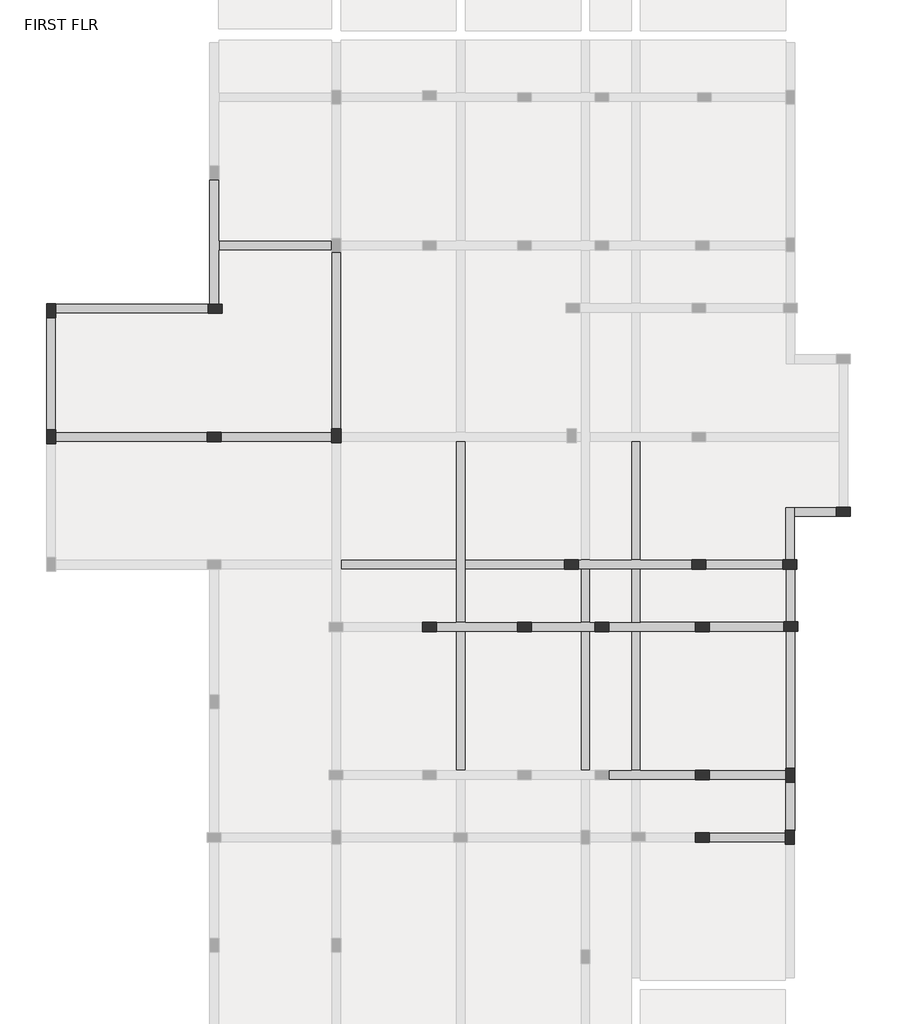
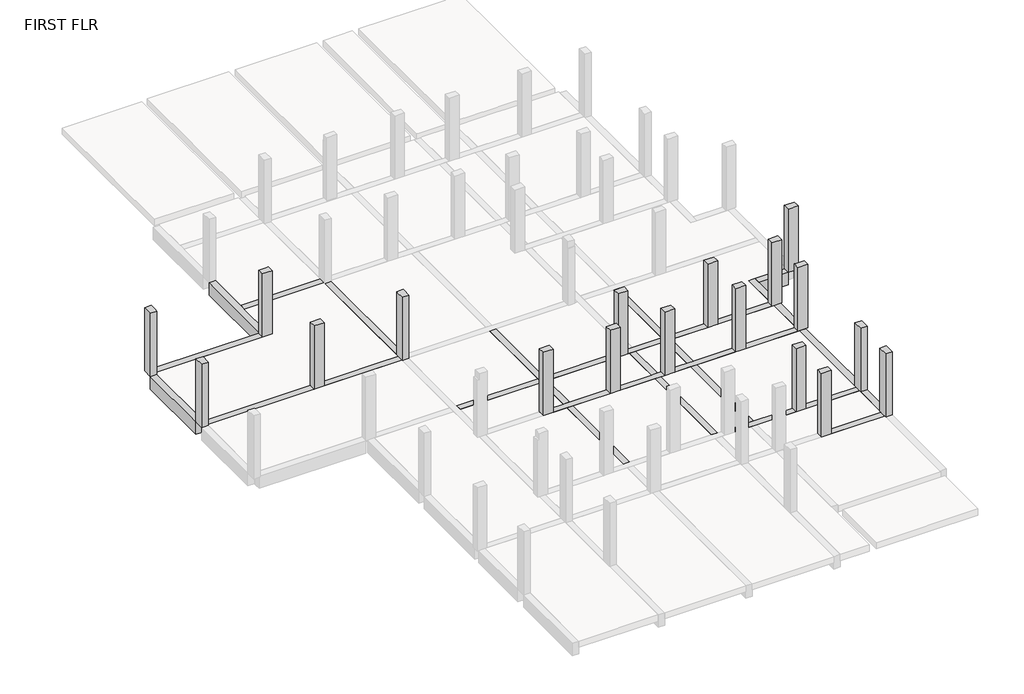
# One storey, part 3 of 5: 30 beams, 18 columns.
"""IFC4 building model written with IfcOpenShell, lengths in millimetres."""

from ifc_helpers import new_model, si_unit, frame, origin, place, context, project, spatial, polyline, outline, extrude, faceted_brep, element, save

model = new_model("IFC4")

# Units and contexts
model_context = context("Model", 3, world=origin())
ifc_project = project(units=[si_unit("LENGTHUNIT", "METRE", prefix="MILLI")], contexts=[model_context])

# Site, building, storey
site = spatial("IfcSite", under=ifc_project)
building = spatial("IfcBuilding", under=site)
storey = spatial("IfcBuildingStorey", under=building, Name="FIRST FLR", Elevation=3000.0)

# Beams
placement = place(None, origin())
element("IfcBeam", 1, ObjectType="M_Concrete-Rectangular Beam : 300 x 600mm", at=placement, inside=storey, context=model_context, shape_type="Brep", body=[
    faceted_brep([(-5888.8105653, 9367.5252033, 3000.0), (-5888.8105653, 5367.5252033, 3000.0), (-5588.8105653, 5367.5252033, 3000.0), (-5588.8105653, 7099.7076276, 3000.0), (-5588.8105653, 7399.7076276, 3000.0), (-5588.8105653, 9367.5252033, 3000.0), (-5888.8105653, 9367.5252033, 2400.0), (-5888.8105653, 5367.5252033, 2400.0), (-5588.8105653, 9367.5252033, 2400.0), (-5588.8105653, 7399.7076276, 2400.0), (-5588.8105653, 7099.7076276, 2400.0), (-5588.8105653, 5367.5252033, 2400.0), (-5588.8105653, 9367.5252033, 2700.0), (-5588.8105653, 5367.5252033, 2700.0)], [[[0, 1, 2, 3, 4, 5]], [[1, 0, 6, 7]], [[7, 6, 8, 9, 10, 11]], [[11, 10, 9, 8, 12, 5, 4, 3, 2, 13]], [[8, 6, 0, 5, 12]], [[2, 1, 7, 11, 13]]]),
])
element("IfcBeam", 2, ObjectType="M_Concrete-Rectangular Beam : 300 x 600mm", at=placement, inside=storey, context=model_context, shape_type="Brep", body=[
    faceted_brep([(-5943.8105653, 5067.6057249, 3000.0), (-5943.8105653, 5367.6057249, 3000.0), (-10828.8105653, 5367.6057249, 3000.0), (-10828.8105653, 5067.6057249, 3000.0), (-5943.8105653, 5367.6057249, 2400.0), (-10828.8105653, 5367.6057249, 2400.0), (-5943.8105653, 5067.6057249, 2400.0), (-10828.8105653, 5067.6057249, 2400.0), (-10828.8105653, 5067.6057249, 2700.0), (-5943.8105653, 5067.6057249, 2700.0)], [[[0, 1, 2, 3]], [[1, 4, 5, 2]], [[4, 6, 7, 5]], [[0, 3, 8, 7, 6, 9]], [[6, 4, 1, 0, 9]], [[3, 2, 5, 7, 8]]]),
])
element("IfcBeam", 3, ObjectType="M_Concrete-Rectangular Beam : 300 x 600mm", at=placement, inside=storey, context=model_context, shape_type="SweptSolid", body=[
    extrude(outline(polyline([(-10828.8105653, 1326.1713929), (-11128.8105653, 1326.1713929), (-11128.8105653, 4932.6057249), (-10828.8105653, 4932.6057249), (-10828.8105653, 1326.1713929)])), frame((0.0, 0.0, 2400.0), z_axis=(0.0, 0.0, 1.0), x_axis=(1.0, 0.0, 0.0)), (0.0, 0.0, 1.0), 600.0),
])
element("IfcBeam", 4, ObjectType="M_Concrete-Rectangular Beam : 300 x 600mm", at=placement, inside=storey, context=model_context, shape_type="SweptSolid", body=[
    extrude(outline(polyline([(12619.1163908, -9982.1078267), (12919.1163908, -9982.1078267), (12919.1163908, -11537.8970059), (12899.1163908, -11537.8970059), (12899.1163908, -11532.8970059), (12619.1163908, -11532.8970059), (12619.1163908, -9982.1078267)])), frame((0.0, 0.0, 2400.0), z_axis=(0.0, 0.0, 1.0), x_axis=(1.0, 0.0, 0.0)), (0.0, 0.0, 1.0), 600.0),
])
element("IfcBeam", 5, ObjectType="M_Concrete-Rectangular Beam : 300 x 600mm", at=placement, inside=storey, context=model_context, shape_type="Brep", body=[
    faceted_brep([(12619.1163908, -5144.3229916, 3000.0), (12919.1163908, -5144.3229916, 3000.0), (12919.1163908, -5144.3229916, 2400.0), (12619.1163908, -5144.3229916, 2400.0), (12619.1163908, -5151.6229916, 3000.0), (12619.1163908, -9532.1078267, 3000.0), (12919.1163908, -9532.1078267, 3000.0), (12919.1163908, -9532.1078267, 2400.0), (12619.1163908, -9532.1078267, 2400.0), (12619.1163908, -5151.6229916, 2400.0), (12619.1163908, -9532.1078267, 2700.0)], [[[0, 1, 2, 3]], [[1, 0, 4, 5, 6]], [[2, 1, 6, 7]], [[3, 2, 7, 8, 9]], [[0, 3, 9, 8, 10, 5, 4]], [[8, 7, 6, 5, 10]]]),
])
element("IfcBeam", 6, ObjectType="M_Concrete-Rectangular Beam : 300 x 600mm", at=placement, inside=storey, context=model_context, shape_type="Brep", body=[
    faceted_brep([(12619.1163908, -4818.9229916, 2400.0), (12919.1163908, -4818.9229916, 2400.0), (12919.1163908, -4818.9229916, 3000.0), (12619.1163908, -4818.9229916, 3000.0), (12619.1163908, -4818.9229916, 2700.0), (12919.1163908, -3139.4535766, 3000.0), (12619.1163908, -3139.4535766, 3000.0), (12919.1163908, -3139.4535766, 2400.0), (12619.1163908, -3139.4535766, 2400.0), (12619.1163908, -3139.4535766, 2700.0)], [[[0, 1, 2, 3, 4]], [[3, 2, 5, 6]], [[2, 1, 7, 5]], [[1, 0, 8, 7]], [[3, 6, 9, 8, 0, 4]], [[6, 5, 7, 8, 9]]]),
])
element("IfcBeam", 7, ObjectType="M_Concrete-Rectangular Beam : 300 x 600mm", at=placement, inside=storey, context=model_context, shape_type="Brep", body=[
    faceted_brep([(12599.1163908, -2839.4535766, 3000.0), (12899.1163908, -2839.4535766, 3000.0), (12899.1163908, -1448.8286071, 3000.0), (12899.1163908, -1148.8286071, 3000.0), (12599.1163908, -1148.8286071, 3000.0), (12899.1163908, -2839.4535766, 2400.0), (12899.1163908, -1448.8286071, 2400.0), (12899.1163908, -1148.8286071, 2400.0), (12899.1163908, -1148.8286071, 2700.0), (12599.1163908, -2839.4535766, 2400.0), (12599.1163908, -1148.8286071, 2400.0), (12599.1163908, -1148.8286071, 2700.0), (12599.1163908, -2839.4535766, 2700.0)], [[[0, 1, 2, 3, 4]], [[1, 5, 6, 7, 8, 3, 2]], [[5, 9, 10, 7, 6]], [[0, 4, 11, 10, 9, 12]], [[9, 5, 1, 0, 12]], [[4, 3, 8, 7, 10, 11]]]),
])
element("IfcBeam", 8, ObjectType="M_Concrete-Rectangular Beam : 300 x 600mm", at=placement, inside=storey, context=model_context, shape_type="Brep", body=[
    faceted_brep([(14244.1163908, -1448.8286071, 3000.0), (14244.1163908, -1148.8286071, 3000.0), (12899.1163908, -1148.8286071, 3000.0), (12899.1163908, -1448.8286071, 3000.0), (14244.1163908, -1148.8286071, 2700.0), (14244.1163908, -1148.8286071, 2400.0), (12899.1163908, -1148.8286071, 2400.0), (12899.1163908, -1148.8286071, 2700.0), (14244.1163908, -1448.8286071, 2400.0), (12899.1163908, -1448.8286071, 2400.0)], [[[0, 1, 2, 3]], [[2, 1, 4, 5, 6, 7]], [[5, 8, 9, 6]], [[8, 0, 3, 9]], [[0, 8, 5, 4, 1]], [[3, 2, 7, 6, 9]]]),
])
element("IfcBeam", 9, ObjectType="M_Concrete-Rectangular Beam : 300 x 600mm", at=placement, inside=storey, context=model_context, shape_type="Brep", body=[
    faceted_brep([(-1671.7865686, 7024.7076276, 3000.0), (-1971.7865686, 7024.7076276, 3000.0), (-1971.7865686, 1366.1713929, 3000.0), (-1671.7865686, 1366.1713929, 3000.0), (-1971.7865686, 7024.7076276, 2700.0), (-1971.7865686, 7024.7076276, 2400.0), (-1971.7865686, 1366.1713929, 2400.0), (-1971.7865686, 1366.1713929, 2700.0), (-1671.7865686, 7024.7076276, 2400.0), (-1671.7865686, 1366.1713929, 2400.0), (-1671.7865686, 1366.1713929, 2700.0), (-1671.7865686, 7024.7076276, 2700.0)], [[[0, 1, 2, 3]], [[2, 1, 4, 5, 6, 7]], [[5, 8, 9, 6]], [[0, 3, 10, 9, 8, 11]], [[1, 0, 11, 8, 5, 4]], [[3, 2, 7, 6, 9, 10]]]),
])
element("IfcBeam", 10, ObjectType="M_Concrete-Rectangular Beam : 300 x 600mm", at=placement, inside=storey, context=model_context, shape_type="Brep", body=[
    faceted_brep([(-1971.7865686, 7099.7076276, 3000.0), (-1971.7865686, 7399.7076276, 3000.0), (-5588.8105653, 7399.7076276, 3000.0), (-5588.8105653, 7099.7076276, 3000.0), (-5588.8105653, 7099.7076276, 2700.0), (-5588.8105653, 7099.7076276, 2400.0), (-1971.7865686, 7099.7076276, 2400.0), (-1971.7865686, 7099.7076276, 2700.0), (-1971.7865686, 7399.7076276, 2400.0), (-5588.8105653, 7399.7076276, 2400.0), (-1971.7865686, 7399.7076276, 2700.0), (-5588.8105653, 7399.7076276, 2700.0)], [[[0, 1, 2, 3]], [[0, 3, 4, 5, 6, 7]], [[8, 6, 5, 9]], [[2, 1, 10, 8, 9, 11]], [[1, 0, 7, 6, 8, 10]], [[3, 2, 11, 9, 5, 4]]]),
])
element("IfcBeam", 11, ObjectType="M_Concrete-Rectangular Beam : 300 x 600mm", at=placement, inside=storey, context=model_context, shape_type="Brep", body=[
    faceted_brep([(-10828.8105653, 1251.1713929, 3000.0), (-10828.8105653, 951.1713929, 3000.0), (-5963.8105653, 951.1713929, 3000.0), (-5963.8105653, 1251.1713929, 3000.0), (-10828.8105653, 951.1713929, 2700.0), (-10828.8105653, 951.1713929, 2400.0), (-5963.8105653, 951.1713929, 2400.0), (-5963.8105653, 951.1713929, 2700.0), (-10828.8105653, 1251.1713929, 2400.0), (-5963.8105653, 1251.1713929, 2400.0), (-5963.8105653, 1251.1713929, 2700.0), (-10828.8105653, 1251.1713929, 2700.0)], [[[0, 1, 2, 3]], [[2, 1, 4, 5, 6, 7]], [[5, 8, 9, 6]], [[0, 3, 10, 9, 8, 11]], [[1, 0, 11, 8, 5, 4]], [[3, 2, 7, 6, 9, 10]]]),
])
element("IfcBeam", 12, ObjectType="M_Concrete-Rectangular Beam : 300 x 600mm", at=placement, inside=storey, context=model_context, shape_type="Brep", body=[
    faceted_brep([(-5513.8105653, 1251.1713929, 3000.0), (-5513.8105653, 951.1713929, 3000.0), (-1971.7865686, 951.1713929, 3000.0), (-1971.7865686, 1251.1713929, 3000.0), (-5513.8105653, 951.1713929, 2700.0), (-5513.8105653, 951.1713929, 2400.0), (-1971.7865686, 951.1713929, 2400.0), (-1971.7865686, 951.1713929, 2700.0), (-5513.8105653, 1251.1713929, 2400.0), (-1971.7865686, 1251.1713929, 2400.0), (-1971.7865686, 1251.1713929, 2700.0), (-5513.8105653, 1251.1713929, 2700.0)], [[[0, 1, 2, 3]], [[2, 1, 4, 5, 6, 7]], [[5, 8, 9, 6]], [[0, 3, 10, 9, 8, 11]], [[1, 0, 11, 8, 5, 4]], [[3, 2, 7, 6, 9, 10]]]),
])
element("IfcBeam", 13, ObjectType="M_Concrete-Rectangular Beam : 300 x 600mm", at=placement, inside=storey, context=model_context, shape_type="Brep", body=[
    faceted_brep([(9601.8679014, -3139.4535766, 3000.0), (9601.8679014, -2839.4535766, 3000.0), (7956.8679014, -2839.4535766, 3000.0), (7656.8679014, -2839.4535766, 3000.0), (6332.5248054, -2839.4535766, 3000.0), (6032.5248054, -2839.4535766, 3000.0), (5967.5248054, -2839.4535766, 3000.0), (5967.5248054, -3139.4535766, 3000.0), (6032.5248054, -3139.4535766, 3000.0), (6332.5248054, -3139.4535766, 3000.0), (7656.8679014, -3139.4535766, 3000.0), (7956.8679014, -3139.4535766, 3000.0), (5967.5248054, -3139.4535766, 2400.0), (6032.5248054, -3139.4535766, 2400.0), (6332.5248054, -3139.4535766, 2400.0), (7656.8679014, -3139.4535766, 2400.0), (7956.8679014, -3139.4535766, 2400.0), (9601.8679014, -3139.4535766, 2400.0), (9601.8679014, -3139.4535766, 2700.0), (5967.5248054, -3139.4535766, 2700.0), (9601.8679014, -2839.4535766, 2400.0), (5967.5248054, -2839.4535766, 2400.0), (6032.5248054, -2839.4535766, 2400.0), (6332.5248054, -2839.4535766, 2400.0), (7656.8679014, -2839.4535766, 2400.0), (7956.8679014, -2839.4535766, 2400.0), (5967.5248054, -2839.4535766, 2700.0), (9601.8679014, -2839.4535766, 2700.0)], [[[0, 1, 2, 3, 4, 5, 6, 7, 8, 9, 10, 11]], [[12, 13, 14, 15, 16, 17, 18, 0, 11, 10, 9, 8, 7, 19]], [[20, 17, 16, 15, 14, 13, 12, 21, 22, 23, 24, 25]], [[20, 25, 24, 23, 22, 21, 26, 6, 5, 4, 3, 2, 1, 27]], [[1, 0, 18, 17, 20, 27]], [[7, 6, 26, 21, 12, 19]]]),
])
element("IfcBeam", 14, ObjectType="M_Concrete-Rectangular Beam : 300 x 600mm", at=placement, inside=storey, context=model_context, shape_type="Brep", body=[
    faceted_brep([(12524.1163908, -3139.4535766, 3000.0), (12524.1163908, -2839.4535766, 3000.0), (10051.8679014, -2839.4535766, 3000.0), (10051.8679014, -3139.4535766, 3000.0), (10051.8679014, -3139.4535766, 2700.0), (10051.8679014, -3139.4535766, 2400.0), (12524.1163908, -3139.4535766, 2400.0), (12524.1163908, -3139.4535766, 2700.0), (12524.1163908, -2839.4535766, 2400.0), (10051.8679014, -2839.4535766, 2400.0), (12524.1163908, -2839.4535766, 2700.0), (10051.8679014, -2839.4535766, 2700.0)], [[[0, 1, 2, 3]], [[0, 3, 4, 5, 6, 7]], [[8, 6, 5, 9]], [[2, 1, 10, 8, 9, 11]], [[1, 0, 7, 6, 8, 10]], [[3, 2, 11, 9, 5, 4]]]),
])
element("IfcBeam", 15, ObjectType="M_Concrete-Rectangular Beam : 300 x 600mm", at=placement, inside=storey, context=model_context, shape_type="Brep", body=[
    faceted_brep([(1399.7296816, -4851.6229916, 3000.0), (1399.7296816, -5151.6229916, 3000.0), (2024.7296816, -5151.6229916, 3000.0), (2324.7296816, -5151.6229916, 3000.0), (3997.5248054, -5151.6229916, 3000.0), (3997.5248054, -4851.6229916, 3000.0), (2324.7296816, -4851.6229916, 3000.0), (2024.7296816, -4851.6229916, 3000.0), (1399.7296816, -5151.6229916, 2400.0), (2024.7296816, -5151.6229916, 2400.0), (2324.7296816, -5151.6229916, 2400.0), (3997.5248054, -5151.6229916, 2400.0), (3997.5248054, -5151.6229916, 2700.0), (1399.7296816, -5151.6229916, 2700.0), (1399.7296816, -4851.6229916, 2400.0), (2024.7296816, -4851.6229916, 2400.0), (2324.7296816, -4851.6229916, 2400.0), (3997.5248054, -4851.6229916, 2400.0), (1399.7296816, -4851.6229916, 2700.0), (3997.5248054, -4851.6229916, 2700.0)], [[[0, 1, 2, 3, 4, 5, 6, 7]], [[8, 9, 10, 11, 12, 4, 3, 2, 1, 13]], [[8, 14, 15, 16, 17, 11, 10, 9]], [[17, 16, 15, 14, 18, 0, 7, 6, 5, 19]], [[1, 0, 18, 14, 8, 13]], [[5, 4, 12, 11, 17, 19]]]),
])
element("IfcBeam", 16, ObjectType="M_Concrete-Rectangular Beam : 300 x 600mm", at=placement, inside=storey, context=model_context, shape_type="Brep", body=[
    faceted_brep([(4447.5248054, -4851.6229916, 3000.0), (4447.5248054, -5151.6229916, 3000.0), (6032.5248054, -5151.6229916, 3000.0), (6332.5248054, -5151.6229916, 3000.0), (6481.8679014, -5151.6229916, 3000.0), (6481.8679014, -4851.6229916, 3000.0), (6332.5248054, -4851.6229916, 3000.0), (6032.5248054, -4851.6229916, 3000.0), (4447.5248054, -5151.6229916, 2400.0), (6032.5248054, -5151.6229916, 2400.0), (6332.5248054, -5151.6229916, 2400.0), (6481.8679014, -5151.6229916, 2400.0), (6481.8679014, -5151.6229916, 2700.0), (4447.5248054, -5151.6229916, 2700.0), (4447.5248054, -4851.6229916, 2400.0), (6032.5248054, -4851.6229916, 2400.0), (6332.5248054, -4851.6229916, 2400.0), (6481.8679014, -4851.6229916, 2400.0), (4447.5248054, -4851.6229916, 2700.0)], [[[0, 1, 2, 3, 4, 5, 6, 7]], [[8, 9, 10, 11, 12, 4, 3, 2, 1, 13]], [[8, 14, 15, 16, 17, 11, 10, 9]], [[17, 16, 15, 14, 18, 0, 7, 6, 5]], [[1, 0, 18, 14, 8, 13]], [[5, 4, 12, 11, 17]]]),
])
element("IfcBeam", 17, ObjectType="M_Concrete-Rectangular Beam : 300 x 600mm", at=placement, inside=storey, context=model_context, shape_type="Brep", body=[
    faceted_brep([(6931.8679014, -4851.6229916, 3000.0), (6931.8679014, -5151.6229916, 3000.0), (7656.8679014, -5151.6229916, 3000.0), (7956.8679014, -5151.6229916, 3000.0), (9721.8679014, -5151.6229916, 3000.0), (9721.8679014, -4851.6229916, 3000.0), (7956.8679014, -4851.6229916, 3000.0), (7656.8679014, -4851.6229916, 3000.0), (6931.8679014, -5151.6229916, 2400.0), (7656.8679014, -5151.6229916, 2400.0), (7956.8679014, -5151.6229916, 2400.0), (9721.8679014, -5151.6229916, 2400.0), (9721.8679014, -5151.6229916, 2700.0), (6931.8679014, -5151.6229916, 2700.0), (6931.8679014, -4851.6229916, 2400.0), (7656.8679014, -4851.6229916, 2400.0), (7956.8679014, -4851.6229916, 2400.0), (9721.8679014, -4851.6229916, 2400.0)], [[[0, 1, 2, 3, 4, 5, 6, 7]], [[8, 9, 10, 11, 12, 4, 3, 2, 1, 13]], [[8, 14, 15, 16, 17, 11, 10, 9]], [[14, 0, 7, 6, 5, 17, 16, 15]], [[1, 0, 14, 8, 13]], [[5, 4, 12, 11, 17]]]),
])
element("IfcBeam", 18, ObjectType="M_Concrete-Rectangular Beam : 300 x 600mm", at=placement, inside=storey, context=model_context, shape_type="Brep", body=[
    faceted_brep([(12599.1163908, -11907.8970059, 3000.0), (12599.1163908, -11607.8970059, 3000.0), (10171.8679014, -11607.8970059, 3000.0), (10171.8679014, -11907.8970059, 3000.0), (10171.8679014, -11907.8970059, 2700.0), (10171.8679014, -11907.8970059, 2400.0), (12599.1163908, -11907.8970059, 2400.0), (12599.1163908, -11907.8970059, 2700.0), (12599.1163908, -11607.8970059, 2400.0), (10171.8679014, -11607.8970059, 2400.0), (12599.1163908, -11607.8970059, 2700.0), (10171.8679014, -11607.8970059, 2700.0)], [[[0, 1, 2, 3]], [[0, 3, 4, 5, 6, 7]], [[8, 6, 5, 9]], [[2, 1, 10, 8, 9, 11]], [[1, 0, 7, 6, 8, 10]], [[3, 2, 11, 9, 5, 4]]]),
])
element("IfcBeam", 19, ObjectType="M_Concrete-Rectangular Beam : 300 x 600mm", at=placement, inside=storey, context=model_context, shape_type="Brep", body=[
    faceted_brep([(6931.8679014, -9607.1078267, 3000.0), (6931.8679014, -9907.1078267, 3000.0), (7656.8679014, -9907.1078267, 3000.0), (7956.8679014, -9907.1078267, 3000.0), (9721.8679014, -9907.1078267, 3000.0), (9721.8679014, -9607.1078267, 3000.0), (7956.8679014, -9607.1078267, 3000.0), (7656.8679014, -9607.1078267, 3000.0), (6931.8679014, -9907.1078267, 2400.0), (7656.8679014, -9907.1078267, 2400.0), (7956.8679014, -9907.1078267, 2400.0), (9721.8679014, -9907.1078267, 2400.0), (9721.8679014, -9907.1078267, 2700.0), (6931.8679014, -9907.1078267, 2700.0), (6931.8679014, -9607.1078267, 2400.0), (7656.8679014, -9607.1078267, 2400.0), (7956.8679014, -9607.1078267, 2400.0), (9721.8679014, -9607.1078267, 2400.0), (6931.8679014, -9607.1078267, 2700.0), (9721.8679014, -9607.1078267, 2700.0)], [[[0, 1, 2, 3, 4, 5, 6, 7]], [[8, 9, 10, 11, 12, 4, 3, 2, 1, 13]], [[8, 14, 15, 16, 17, 11, 10, 9]], [[17, 16, 15, 14, 18, 0, 7, 6, 5, 19]], [[1, 0, 18, 14, 8, 13]], [[5, 4, 12, 11, 17, 19]]]),
])
element("IfcBeam", 20, ObjectType="M_Concrete-Rectangular Beam : 300 x 600mm", at=placement, inside=storey, context=model_context, shape_type="Brep", body=[
    faceted_brep([(10171.8679014, -9607.1078267, 3000.0), (10171.8679014, -9907.1078267, 3000.0), (12599.1163908, -9907.1078267, 3000.0), (12619.1163908, -9907.1078267, 3000.0), (12619.1163908, -9607.1078267, 3000.0), (10171.8679014, -9907.1078267, 2400.0), (12619.1163908, -9907.1078267, 2400.0), (10171.8679014, -9907.1078267, 2700.0), (10171.8679014, -9607.1078267, 2400.0), (12619.1163908, -9607.1078267, 2400.0), (12619.1163908, -9607.1078267, 2700.0), (10171.8679014, -9607.1078267, 2700.0)], [[[0, 1, 2, 3, 4]], [[5, 6, 3, 2, 1, 7]], [[5, 8, 9, 6]], [[0, 4, 10, 9, 8, 11]], [[1, 0, 11, 8, 5, 7]], [[4, 3, 6, 9, 10]]]),
])
element("IfcBeam", 21, ObjectType="M_Concrete-Rectangular Beam : 300 x 600mm", at=placement, inside=storey, context=model_context, shape_type="Brep", body=[
    faceted_brep([(-1671.7865686, -2839.4535766, 3000.0), (-1671.7865686, -3139.4535766, 3000.0), (2024.7296816, -3139.4535766, 3000.0), (2024.7296816, -2839.4535766, 3000.0), (-1671.7865686, -3139.4535766, 2700.0), (-1671.7865686, -3139.4535766, 2400.0), (2024.7296816, -3139.4535766, 2400.0), (2024.7296816, -3139.4535766, 2700.0), (-1671.7865686, -2839.4535766, 2400.0), (2024.7296816, -2839.4535766, 2400.0), (2024.7296816, -2839.4535766, 2700.0), (-1671.7865686, -2839.4535766, 2700.0)], [[[0, 1, 2, 3]], [[2, 1, 4, 5, 6, 7]], [[5, 8, 9, 6]], [[0, 3, 10, 9, 8, 11]], [[1, 0, 11, 8, 5, 4]], [[3, 2, 7, 6, 9, 10]]]),
])
element("IfcBeam", 22, ObjectType="M_Concrete-Rectangular Beam : 300 x 600mm", at=placement, inside=storey, context=model_context, shape_type="Brep", body=[
    faceted_brep([(6332.5248054, -3139.4535766, 3000.0), (6032.5248054, -3139.4535766, 3000.0), (6032.5248054, -4851.6229916, 3000.0), (6332.5248054, -4851.6229916, 3000.0), (6032.5248054, -3139.4535766, 2700.0), (6032.5248054, -3139.4535766, 2400.0), (6032.5248054, -4851.6229916, 2400.0), (6032.5248054, -4851.6229916, 2700.0), (6332.5248054, -3139.4535766, 2400.0), (6332.5248054, -4851.6229916, 2400.0), (6332.5248054, -3139.4535766, 2700.0), (6332.5248054, -4851.6229916, 2700.0)], [[[0, 1, 2, 3]], [[2, 1, 4, 5, 6, 7]], [[5, 8, 9, 6]], [[8, 10, 0, 3, 11, 9]], [[1, 0, 10, 8, 5, 4]], [[3, 2, 7, 6, 9, 11]]]),
])
element("IfcBeam", 23, ObjectType="M_Concrete-Rectangular Beam : 300 x 600mm", at=placement, inside=storey, context=model_context, shape_type="Brep", body=[
    faceted_brep([(7956.8679014, -3139.4535766, 3000.0), (7656.8679014, -3139.4535766, 3000.0), (7656.8679014, -4851.6229916, 3000.0), (7956.8679014, -4851.6229916, 3000.0), (7956.8679014, -4831.6229916, 3000.0), (7656.8679014, -3139.4535766, 2700.0), (7656.8679014, -3139.4535766, 2400.0), (7656.8679014, -4851.6229916, 2400.0), (7656.8679014, -4851.6229916, 2700.0), (7956.8679014, -3139.4535766, 2400.0), (7956.8679014, -4851.6229916, 2400.0), (7956.8679014, -3139.4535766, 2700.0)], [[[0, 1, 2, 3, 4]], [[1, 5, 6, 7, 8, 2]], [[6, 9, 10, 7]], [[10, 9, 11, 0, 4, 3]], [[1, 0, 11, 9, 6, 5]], [[3, 2, 8, 7, 10]]]),
])
element("IfcBeam", 24, ObjectType="M_Concrete-Rectangular Beam : 300 x 600mm", at=placement, inside=storey, context=model_context, shape_type="Brep", body=[
    faceted_brep([(2324.7296816, -5151.6229916, 3000.0), (2024.7296816, -5151.6229916, 3000.0), (2024.7296816, -9607.1078267, 3000.0), (2324.7296816, -9607.1078267, 3000.0), (2024.7296816, -5151.6229916, 2700.0), (2024.7296816, -5151.6229916, 2400.0), (2024.7296816, -9607.1078267, 2400.0), (2024.7296816, -9607.1078267, 2700.0), (2324.7296816, -5151.6229916, 2400.0), (2324.7296816, -9607.1078267, 2400.0), (2324.7296816, -9607.1078267, 2700.0), (2324.7296816, -5151.6229916, 2700.0)], [[[0, 1, 2, 3]], [[2, 1, 4, 5, 6, 7]], [[5, 8, 9, 6]], [[0, 3, 10, 9, 8, 11]], [[1, 0, 11, 8, 5, 4]], [[3, 2, 7, 6, 9, 10]]]),
])
element("IfcBeam", 25, ObjectType="M_Concrete-Rectangular Beam : 300 x 600mm", at=placement, inside=storey, context=model_context, shape_type="Brep", body=[
    faceted_brep([(6332.5248054, -5151.6229916, 3000.0), (6032.5248054, -5151.6229916, 3000.0), (6032.5248054, -9607.1078267, 3000.0), (6332.5248054, -9607.1078267, 3000.0), (6032.5248054, -5151.6229916, 2700.0), (6032.5248054, -5151.6229916, 2400.0), (6032.5248054, -9607.1078267, 2400.0), (6032.5248054, -9607.1078267, 2700.0), (6332.5248054, -5151.6229916, 2400.0), (6332.5248054, -9607.1078267, 2400.0), (6332.5248054, -9607.1078267, 2700.0), (6332.5248054, -5151.6229916, 2700.0)], [[[0, 1, 2, 3]], [[2, 1, 4, 5, 6, 7]], [[5, 8, 9, 6]], [[0, 3, 10, 9, 8, 11]], [[1, 0, 11, 8, 5, 4]], [[3, 2, 7, 6, 9, 10]]]),
])
element("IfcBeam", 26, ObjectType="M_Concrete-Rectangular Beam : 300 x 600mm", at=placement, inside=storey, context=model_context, shape_type="Brep", body=[
    faceted_brep([(7956.8679014, -5151.6229916, 3000.0), (7656.8679014, -5151.6229916, 3000.0), (7656.8679014, -9607.1078267, 3000.0), (7956.8679014, -9607.1078267, 3000.0), (7656.8679014, -5151.6229916, 2700.0), (7656.8679014, -5151.6229916, 2400.0), (7656.8679014, -9607.1078267, 2400.0), (7656.8679014, -9607.1078267, 2700.0), (7956.8679014, -5151.6229916, 2400.0), (7956.8679014, -9607.1078267, 2400.0), (7956.8679014, -9607.1078267, 2700.0), (7956.8679014, -5151.6229916, 2700.0)], [[[0, 1, 2, 3]], [[2, 1, 4, 5, 6, 7]], [[5, 8, 9, 6]], [[0, 3, 10, 9, 8, 11]], [[1, 0, 11, 8, 5, 4]], [[3, 2, 7, 6, 9, 10]]]),
])
element("IfcBeam", 27, ObjectType="M_Concrete-Rectangular Beam : 300 x 600mm", at=placement, inside=storey, context=model_context, shape_type="Brep", body=[
    faceted_brep([(2024.7296816, -4851.6229916, 3000.0), (2324.7296816, -4851.6229916, 3000.0), (2324.7296816, -3139.4535766, 3000.0), (2324.7296816, -2839.4535766, 3000.0), (2324.7296816, 951.1713929, 3000.0), (2024.7296816, 951.1713929, 3000.0), (2024.7296816, -2839.4535766, 3000.0), (2024.7296816, -3139.4535766, 3000.0), (2024.7296816, 951.1713929, 2400.0), (2024.7296816, -2839.4535766, 2400.0), (2024.7296816, -3139.4535766, 2400.0), (2024.7296816, -4851.6229916, 2400.0), (2024.7296816, -4851.6229916, 2700.0), (2024.7296816, 951.1713929, 2700.0), (2324.7296816, -4851.6229916, 2400.0), (2324.7296816, 951.1713929, 2400.0), (2324.7296816, -2839.4535766, 2400.0), (2324.7296816, -3139.4535766, 2400.0), (2324.7296816, 951.1713929, 2700.0), (2324.7296816, -4851.6229916, 2700.0)], [[[0, 1, 2, 3, 4, 5, 6, 7]], [[8, 9, 10, 11, 12, 0, 7, 6, 5, 13]], [[14, 11, 10, 9, 8, 15, 16, 17]], [[14, 17, 16, 15, 18, 4, 3, 2, 1, 19]], [[1, 0, 12, 11, 14, 19]], [[5, 4, 18, 15, 8, 13]]]),
])
element("IfcBeam", 28, ObjectType="M_Concrete-Rectangular Beam : 300 x 600mm", at=placement, inside=storey, context=model_context, shape_type="Brep", body=[
    faceted_brep([(5517.5248054, -3139.4535766, 3000.0), (5517.5248054, -2839.4535766, 3000.0), (2324.7296816, -2839.4535766, 3000.0), (2324.7296816, -3139.4535766, 3000.0), (2324.7296816, -3139.4535766, 2700.0), (2324.7296816, -3139.4535766, 2400.0), (5517.5248054, -3139.4535766, 2400.0), (5517.5248054, -3139.4535766, 2700.0), (5517.5248054, -2839.4535766, 2400.0), (2324.7296816, -2839.4535766, 2400.0), (5517.5248054, -2839.4535766, 2700.0), (2324.7296816, -2839.4535766, 2700.0)], [[[0, 1, 2, 3]], [[0, 3, 4, 5, 6, 7]], [[8, 6, 5, 9]], [[2, 1, 10, 8, 9, 11]], [[1, 0, 7, 6, 8, 10]], [[3, 2, 11, 9, 5, 4]]]),
])
element("IfcBeam", 29, ObjectType="M_Concrete-Rectangular Beam : 300 x 600mm", at=placement, inside=storey, context=model_context, shape_type="Brep", body=[
    faceted_brep([(7656.8679014, -2839.4535766, 3000.0), (7956.8679014, -2839.4535766, 3000.0), (7956.8679014, 951.1713929, 3000.0), (7656.8679014, 951.1713929, 3000.0), (7656.8679014, 951.1713929, 2700.0), (7656.8679014, 951.1713929, 2400.0), (7656.8679014, -2839.4535766, 2400.0), (7656.8679014, -2839.4535766, 2700.0), (7956.8679014, -2839.4535766, 2400.0), (7956.8679014, 951.1713929, 2400.0), (7956.8679014, -2839.4535766, 2700.0), (7956.8679014, 951.1713929, 2700.0)], [[[0, 1, 2, 3]], [[0, 3, 4, 5, 6, 7]], [[8, 6, 5, 9]], [[2, 1, 10, 8, 9, 11]], [[1, 0, 7, 6, 8, 10]], [[3, 2, 11, 9, 5, 4]]]),
])
element("IfcBeam", 30, ObjectType="M_Concrete-Rectangular Beam : 300 x 600mm", at=placement, inside=storey, context=model_context, shape_type="Brep", body=[
    faceted_brep([(10171.8679014, -4851.6229916, 3000.0), (10171.8679014, -5151.6229916, 3000.0), (12619.1163908, -5151.6229916, 3000.0), (12619.1163908, -5144.3229916, 3000.0), (12919.1163908, -5144.3229916, 3000.0), (12919.1163908, -5131.6229916, 3000.0), (12564.1163908, -5131.6229916, 3000.0), (12564.1163908, -4851.6229916, 3000.0), (10171.8679014, -5151.6229916, 2700.0), (10171.8679014, -5151.6229916, 2400.0), (12619.1163908, -5151.6229916, 2400.0), (12619.1163908, -5151.6229916, 2700.0), (10171.8679014, -4851.6229916, 2400.0), (12564.1163908, -4851.6229916, 2400.0), (12564.1163908, -5131.6229916, 2400.0), (12919.1163908, -5131.6229916, 2400.0), (12919.1163908, -5144.3229916, 2400.0), (12619.1163908, -5144.3229916, 2400.0)], [[[0, 1, 2, 3, 4, 5, 6, 7]], [[2, 1, 8, 9, 10, 11]], [[9, 12, 13, 14, 15, 16, 17, 10]], [[12, 0, 7, 13]], [[4, 16, 15, 5]], [[1, 0, 12, 9, 8]], [[3, 17, 16, 4]], [[17, 3, 2, 11, 10]], [[14, 6, 5, 15]], [[6, 14, 13, 7]]]),
])

# Columns
element("IfcColumn", 31, ObjectType="M_Concrete-Rectangular-Column : 300 x 450mm", at=placement, inside=storey, context=model_context, shape_type="Brep", body=[
    faceted_brep([(-5943.8105653, 5367.6057249, 3000.0), (-5493.8105653, 5367.6057249, 3000.0), (-5493.8105653, 5067.6057249, 3000.0), (-5943.8105653, 5067.6057249, 3000.0), (-5943.8105653, 5367.6057249, 6048.0), (-5588.8105653, 5367.6057249, 6048.0), (-5493.8105653, 5367.6057249, 6048.0), (-5493.8105653, 5367.6057249, 5748.0), (-5493.8105653, 5067.6057249, 6048.0), (-5493.8105653, 5067.6057249, 5748.0), (-5943.8105653, 5067.6057249, 6048.0), (-5943.8105653, 5067.6057249, 5748.0)], [[[0, 1, 2, 3]], [[1, 0, 4, 5, 6, 7]], [[2, 1, 7, 6, 8, 9]], [[3, 2, 9, 8, 10, 11]], [[0, 3, 11, 10, 4]], [[8, 6, 5, 4, 10]]]),
])
element("IfcColumn", 32, ObjectType="M_Concrete-Rectangular-Column : 300 x 450mm", at=placement, inside=storey, context=model_context, shape_type="Brep", body=[
    faceted_brep([(-10828.8105653, 5382.6057249, 3000.0), (-10828.8105653, 4932.6057249, 3000.0), (-11128.8105653, 4932.6057249, 3000.0), (-11128.8105653, 5382.6057249, 3000.0), (-10828.8105653, 5382.6057249, 6048.0), (-10828.8105653, 5067.6057249, 6048.0), (-10828.8105653, 4932.6057249, 6048.0), (-11128.8105653, 4932.6057249, 6048.0), (-11128.8105653, 5382.6057249, 6048.0)], [[[0, 1, 2, 3]], [[4, 5, 6, 1, 0]], [[6, 7, 2, 1]], [[7, 8, 3, 2]], [[8, 4, 0, 3]], [[4, 8, 7, 6, 5]]]),
])
element("IfcColumn", 33, ObjectType="M_Concrete-Rectangular-Column : 300 x 450mm", at=placement, inside=storey, context=model_context, shape_type="Brep", body=[
    faceted_brep([(-11128.8105653, 876.1713929, 3000.0), (-11128.8105653, 1326.1713929, 3000.0), (-10828.8105653, 1326.1713929, 3000.0), (-10828.8105653, 876.1713929, 3000.0), (-11128.8105653, 876.1713929, 6048.0), (-11128.8105653, 1326.1713929, 6048.0), (-10828.8105653, 1326.1713929, 6048.0), (-10828.8105653, 1251.1713929, 6048.0), (-10828.8105653, 951.1713929, 6048.0), (-10828.8105653, 876.1713929, 6048.0)], [[[0, 1, 2, 3]], [[4, 5, 1, 0]], [[5, 6, 2, 1]], [[6, 7, 8, 9, 3, 2]], [[9, 4, 0, 3]], [[4, 9, 8, 7, 6, 5]]]),
])
element("IfcColumn", 34, ObjectType="M_Concrete-Rectangular-Column : 300 x 450mm", at=placement, inside=storey, context=model_context, shape_type="Brep", body=[
    faceted_brep([(-5513.8105653, 951.1713929, 3000.0), (-5963.8105653, 951.1713929, 3000.0), (-5963.8105653, 1251.1713929, 3000.0), (-5513.8105653, 1251.1713929, 3000.0), (-5513.8105653, 951.1713929, 5748.0), (-5513.8105653, 951.1713929, 6048.0), (-5963.8105653, 951.1713929, 6048.0), (-5963.8105653, 951.1713929, 5748.0), (-5963.8105653, 1251.1713929, 6048.0), (-5963.8105653, 1251.1713929, 5748.0), (-5513.8105653, 1251.1713929, 6048.0), (-5513.8105653, 1251.1713929, 5748.0)], [[[0, 1, 2, 3]], [[1, 0, 4, 5, 6, 7]], [[2, 1, 7, 6, 8, 9]], [[3, 2, 9, 8, 10, 11]], [[0, 3, 11, 10, 5, 4]], [[6, 5, 10, 8]]]),
])
element("IfcColumn", 35, ObjectType="M_Concrete-Rectangular-Column : 300 x 450mm", at=placement, inside=storey, context=model_context, shape_type="Brep", body=[
    faceted_brep([(-1671.7865686, 1366.1713929, 3000.0), (-1671.7865686, 916.1713929, 3000.0), (-1971.7865686, 916.1713929, 3000.0), (-1971.7865686, 1366.1713929, 3000.0), (-1671.7865686, 1366.1713929, 5748.0), (-1671.7865686, 1366.1713929, 6048.0), (-1671.7865686, 1251.1713929, 6048.0), (-1671.7865686, 951.1713929, 6048.0), (-1671.7865686, 916.1713929, 6048.0), (-1671.7865686, 916.1713929, 5748.0), (-1971.7865686, 916.1713929, 6048.0), (-1971.7865686, 916.1713929, 5748.0), (-1971.7865686, 951.1713929, 6048.0), (-1971.7865686, 1251.1713929, 6048.0), (-1971.7865686, 1366.1713929, 6048.0), (-1971.7865686, 1366.1713929, 5748.0)], [[[0, 1, 2, 3]], [[1, 0, 4, 5, 6, 7, 8, 9]], [[2, 1, 9, 8, 10, 11]], [[3, 2, 11, 10, 12, 13, 14, 15]], [[0, 3, 15, 14, 5, 4]], [[10, 8, 7, 6, 5, 14, 13, 12]]]),
])
element("IfcColumn", 36, ObjectType="M_Concrete-Rectangular-Column : 300 x 450mm", at=placement, inside=storey, context=model_context, shape_type="Brep", body=[
    faceted_brep([(14244.1163908, -1148.8286071, 3000.0), (14694.1163908, -1148.8286071, 3000.0), (14694.1163908, -1448.8286071, 3000.0), (14244.1163908, -1448.8286071, 3000.0), (14244.1163908, -1148.8286071, 5748.0), (14244.1163908, -1148.8286071, 6048.0), (14319.1163908, -1148.8286071, 6048.0), (14694.1163908, -1148.8286071, 6048.0), (14694.1163908, -1448.8286071, 6048.0), (14244.1163908, -1448.8286071, 6048.0)], [[[0, 1, 2, 3]], [[1, 0, 4, 5, 6, 7]], [[2, 1, 7, 8]], [[3, 2, 8, 9]], [[0, 3, 9, 5, 4]], [[8, 7, 6, 5, 9]]]),
])
element("IfcColumn", 37, ObjectType="M_Concrete-Rectangular-Column : 300 x 450mm", at=placement, inside=storey, context=model_context, shape_type="Brep", body=[
    faceted_brep([(12524.1163908, -2839.4535766, 3000.0), (12974.1163908, -2839.4535766, 3000.0), (12974.1163908, -3139.4535766, 3000.0), (12524.1163908, -3139.4535766, 3000.0), (12524.1163908, -2839.4535766, 5748.0), (12524.1163908, -2839.4535766, 6048.0), (12599.1163908, -2839.4535766, 6048.0), (12974.1163908, -2839.4535766, 6048.0), (12974.1163908, -3139.4535766, 6048.0), (12619.1163908, -3139.4535766, 6048.0), (12524.1163908, -3139.4535766, 6048.0), (12524.1163908, -3139.4535766, 5748.0)], [[[0, 1, 2, 3]], [[1, 0, 4, 5, 6, 7]], [[2, 1, 7, 8]], [[3, 2, 8, 9, 10, 11]], [[0, 3, 11, 10, 5, 4]], [[8, 7, 6, 5, 10, 9]]]),
])
element("IfcColumn", 38, ObjectType="M_Concrete-Rectangular-Column : 300 x 450mm", at=placement, inside=storey, context=model_context, shape_type="Brep", body=[
    faceted_brep([(9601.8679014, -2839.4535766, 3000.0), (10051.8679014, -2839.4535766, 3000.0), (10051.8679014, -3139.4535766, 3000.0), (9601.8679014, -3139.4535766, 3000.0), (9601.8679014, -2839.4535766, 5748.0), (9601.8679014, -2839.4535766, 6048.0), (10051.8679014, -2839.4535766, 6048.0), (10051.8679014, -2839.4535766, 5748.0), (10051.8679014, -3139.4535766, 6048.0), (10051.8679014, -3139.4535766, 5748.0), (9601.8679014, -3139.4535766, 6048.0), (9601.8679014, -3139.4535766, 5748.0)], [[[0, 1, 2, 3]], [[1, 0, 4, 5, 6, 7]], [[2, 1, 7, 6, 8, 9]], [[3, 2, 9, 8, 10, 11]], [[0, 3, 11, 10, 5, 4]], [[6, 5, 10, 8]]]),
])
element("IfcColumn", 39, ObjectType="M_Concrete-Rectangular-Column : 300 x 450mm", at=placement, inside=storey, context=model_context, shape_type="Brep", body=[
    faceted_brep([(5517.5248054, -2839.4535766, 3000.0), (5967.5248054, -2839.4535766, 3000.0), (5967.5248054, -3139.4535766, 3000.0), (5517.5248054, -3139.4535766, 3000.0), (5517.5248054, -2839.4535766, 5748.0), (5517.5248054, -2839.4535766, 6048.0), (5967.5248054, -2839.4535766, 6048.0), (5967.5248054, -2839.4535766, 5748.0), (5967.5248054, -3139.4535766, 6048.0), (5967.5248054, -3139.4535766, 5748.0), (5517.5248054, -3139.4535766, 6048.0), (5517.5248054, -3139.4535766, 5748.0)], [[[0, 1, 2, 3]], [[1, 0, 4, 5, 6, 7]], [[2, 1, 7, 6, 8, 9]], [[3, 2, 9, 8, 10, 11]], [[0, 3, 11, 10, 5, 4]], [[6, 5, 10, 8]]]),
])
element("IfcColumn", 40, ObjectType="M_Concrete-Rectangular-Column : 300 x 450mm", at=placement, inside=storey, context=model_context, shape_type="Brep", body=[
    faceted_brep([(1399.7296816, -5151.6229916, 3000.0), (949.7296816, -5151.6229916, 3000.0), (949.7296816, -4851.6229916, 3000.0), (1399.7296816, -4851.6229916, 3000.0), (1399.7296816, -5151.6229916, 5748.0), (1399.7296816, -5151.6229916, 6048.0), (949.7296816, -5151.6229916, 6048.0), (949.7296816, -5151.6229916, 5748.0), (949.7296816, -4851.6229916, 6048.0), (949.7296816, -4851.6229916, 5748.0), (1399.7296816, -4851.6229916, 6048.0), (1399.7296816, -4851.6229916, 5748.0)], [[[0, 1, 2, 3]], [[1, 0, 4, 5, 6, 7]], [[2, 1, 7, 6, 8, 9]], [[3, 2, 9, 8, 10, 11]], [[0, 3, 11, 10, 5, 4]], [[6, 5, 10, 8]]]),
])
element("IfcColumn", 41, ObjectType="M_Concrete-Rectangular-Column : 300 x 450mm", at=placement, inside=storey, context=model_context, shape_type="Brep", body=[
    faceted_brep([(4447.5248054, -5151.6229916, 3000.0), (3997.5248054, -5151.6229916, 3000.0), (3997.5248054, -4851.6229916, 3000.0), (4447.5248054, -4851.6229916, 3000.0), (4447.5248054, -5151.6229916, 5748.0), (4447.5248054, -5151.6229916, 6048.0), (3997.5248054, -5151.6229916, 6048.0), (3997.5248054, -5151.6229916, 5748.0), (3997.5248054, -4851.6229916, 6048.0), (3997.5248054, -4851.6229916, 5748.0), (4447.5248054, -4851.6229916, 6048.0), (4447.5248054, -4851.6229916, 5748.0)], [[[0, 1, 2, 3]], [[1, 0, 4, 5, 6, 7]], [[2, 1, 7, 6, 8, 9]], [[3, 2, 9, 8, 10, 11]], [[0, 3, 11, 10, 5, 4]], [[6, 5, 10, 8]]]),
])
element("IfcColumn", 42, ObjectType="M_Concrete-Rectangular-Column : 300 x 450mm", at=placement, inside=storey, context=model_context, shape_type="Brep", body=[
    faceted_brep([(6931.8679014, -5151.6229916, 3000.0), (6481.8679014, -5151.6229916, 3000.0), (6481.8679014, -4851.6229916, 3000.0), (6931.8679014, -4851.6229916, 3000.0), (6931.8679014, -5151.6229916, 5748.0), (6931.8679014, -5151.6229916, 6048.0), (6481.8679014, -5151.6229916, 6048.0), (6481.8679014, -5151.6229916, 5748.0), (6481.8679014, -4851.6229916, 6048.0), (6931.8679014, -4851.6229916, 6048.0)], [[[0, 1, 2, 3]], [[1, 0, 4, 5, 6, 7]], [[2, 1, 7, 6, 8]], [[3, 2, 8, 9]], [[0, 3, 9, 5, 4]], [[6, 5, 9, 8]]]),
])
element("IfcColumn", 43, ObjectType="M_Concrete-Rectangular-Column : 300 x 450mm", at=placement, inside=storey, context=model_context, shape_type="Brep", body=[
    faceted_brep([(10171.8679014, -5151.6229916, 3000.0), (9721.8679014, -5151.6229916, 3000.0), (9721.8679014, -4851.6229916, 3000.0), (10171.8679014, -4851.6229916, 3000.0), (10171.8679014, -5151.6229916, 5748.0), (10171.8679014, -5151.6229916, 6048.0), (9721.8679014, -5151.6229916, 6048.0), (9721.8679014, -5151.6229916, 5748.0), (9721.8679014, -4851.6229916, 6048.0), (10171.8679014, -4851.6229916, 6048.0)], [[[0, 1, 2, 3]], [[1, 0, 4, 5, 6, 7]], [[2, 1, 7, 6, 8]], [[3, 2, 8, 9]], [[0, 3, 9, 5, 4]], [[6, 5, 9, 8]]]),
])
element("IfcColumn", 44, ObjectType="M_Concrete-Rectangular-Column : 300 x 450mm", at=placement, inside=storey, context=model_context, shape_type="Brep", body=[
    faceted_brep([(13014.1163908, -5131.6229916, 3000.0), (12564.1163908, -5131.6229916, 3000.0), (12564.1163908, -4831.6229916, 3000.0), (13014.1163908, -4831.6229916, 3000.0), (13014.1163908, -5131.6229916, 6048.0), (12564.1163908, -5131.6229916, 6048.0), (12564.1163908, -4831.6229916, 6048.0), (12564.1163908, -4831.6229916, 5748.0), (12619.1163908, -4831.6229916, 6048.0), (13014.1163908, -4831.6229916, 6048.0)], [[[0, 1, 2, 3]], [[1, 0, 4, 5]], [[2, 1, 5, 6, 7]], [[3, 2, 7, 6, 8, 9]], [[0, 3, 9, 4]], [[5, 4, 9, 8, 6]]]),
])
element("IfcColumn", 45, ObjectType="M_Concrete-Rectangular-Column : 300 x 450mm", at=placement, inside=storey, context=model_context, shape_type="Brep", body=[
    faceted_brep([(10171.8679014, -9907.1078267, 3000.0), (9721.8679014, -9907.1078267, 3000.0), (9721.8679014, -9607.1078267, 3000.0), (10171.8679014, -9607.1078267, 3000.0), (10171.8679014, -9907.1078267, 5748.0), (10171.8679014, -9907.1078267, 6048.0), (9721.8679014, -9907.1078267, 6048.0), (9721.8679014, -9907.1078267, 5748.0), (9721.8679014, -9607.1078267, 6048.0), (9721.8679014, -9607.1078267, 5748.0), (10171.8679014, -9607.1078267, 6048.0), (10171.8679014, -9607.1078267, 5748.0)], [[[0, 1, 2, 3]], [[1, 0, 4, 5, 6, 7]], [[2, 1, 7, 6, 8, 9]], [[3, 2, 9, 8, 10, 11]], [[0, 3, 11, 10, 5, 4]], [[6, 5, 10, 8]]]),
])
element("IfcColumn", 46, ObjectType="M_Concrete-Rectangular-Column : 300 x 450mm", at=placement, inside=storey, context=model_context, shape_type="Brep", body=[
    faceted_brep([(12919.1163908, -9532.1078267, 3000.0), (12919.1163908, -9982.1078267, 3000.0), (12619.1163908, -9982.1078267, 3000.0), (12619.1163908, -9532.1078267, 3000.0), (12919.1163908, -9532.1078267, 6048.0), (12919.1163908, -9982.1078267, 6048.0), (12619.1163908, -9982.1078267, 6048.0), (12619.1163908, -9607.1078267, 6048.0), (12619.1163908, -9532.1078267, 6048.0), (12619.1163908, -9532.1078267, 5748.0)], [[[0, 1, 2, 3]], [[1, 0, 4, 5]], [[2, 1, 5, 6]], [[3, 2, 6, 7, 8, 9]], [[0, 3, 9, 8, 4]], [[5, 4, 8, 7, 6]]]),
])
element("IfcColumn", 47, ObjectType="M_Concrete-Rectangular-Column : 300 x 450mm", at=placement, inside=storey, context=model_context, shape_type="Brep", body=[
    faceted_brep([(12899.1163908, -11532.8970059, 3000.0), (12899.1163908, -11982.8970059, 3000.0), (12599.1163908, -11982.8970059, 3000.0), (12599.1163908, -11532.8970059, 3000.0), (12899.1163908, -11532.8970059, 6048.0), (12899.1163908, -11982.8970059, 6048.0), (12599.1163908, -11982.8970059, 6048.0), (12599.1163908, -11982.8970059, 5748.0), (12599.1163908, -11907.8970059, 6048.0), (12599.1163908, -11607.8970059, 6048.0), (12599.1163908, -11532.8970059, 6048.0), (12599.1163908, -11532.8970059, 5748.0)], [[[0, 1, 2, 3]], [[1, 0, 4, 5]], [[2, 1, 5, 6, 7]], [[3, 2, 7, 6, 8, 9, 10, 11]], [[0, 3, 11, 10, 4]], [[5, 4, 10, 9, 8, 6]]]),
])
element("IfcColumn", 48, ObjectType="M_Concrete-Rectangular-Column : 300 x 450mm", at=placement, inside=storey, context=model_context, shape_type="Brep", body=[
    faceted_brep([(9721.8679014, -11607.8970059, 3000.0), (10171.8679014, -11607.8970059, 3000.0), (10171.8679014, -11907.8970059, 3000.0), (9721.8679014, -11907.8970059, 3000.0), (9721.8679014, -11607.8970059, 5748.0), (9721.8679014, -11607.8970059, 6048.0), (10171.8679014, -11607.8970059, 6048.0), (10171.8679014, -11607.8970059, 5748.0), (10171.8679014, -11907.8970059, 6048.0), (10171.8679014, -11907.8970059, 5748.0), (9721.8679014, -11907.8970059, 6048.0), (9721.8679014, -11907.8970059, 5748.0)], [[[0, 1, 2, 3]], [[1, 0, 4, 5, 6, 7]], [[2, 1, 7, 6, 8, 9]], [[3, 2, 9, 8, 10, 11]], [[0, 3, 11, 10, 5, 4]], [[6, 5, 10, 8]]]),
])

save(model, "model.ifc")

# Revit data of these elements
# Type "M_Concrete-Rectangular Beam : 300 x 600mm"
#   Length [instance default] = 1524 mm
#   b = 300 mm
#   h = 600 mm
#   Structural Material [instance default] = Concrete, Cast-in-Place gray
#   Assembly Code = ""
# Type "M_Concrete-Rectangular-Column : 300 x 450mm"
#   b = 300 mm
#   h = 450 mm
#   Structural Material [instance default] = Concrete, Cast-in-Place gray
# Elements 1, 2, 3, 4, 5, 6, 7, 8, 9, 10, 11, 12, 13, 14, 15, 16, 17, 18, 19, 20, 30 (IfcBeam, "M_Concrete-Rectangular Beam : 300 x 600mm")
#   Structural Material = Concrete, Cast-in-Place gray
#   Phase Created = New Construction
#   Materials on its faces: "Concrete, Cast-in-Place gray"
# Elements 21, 22, 23, 24, 25, 26, 27, 28, 29 (IfcBeam, "M_Concrete-Rectangular Beam : 300 x 600mm")
#   Phase Created = New Construction
#   Materials on its faces: "Concrete, Cast-in-Place gray"
# Elements 31, 32, 33, 34, 35, 36, 37, 38, 39, 40, 41, 42, 43, 44, 45, 46, 47, 48 (IfcColumn, "M_Concrete-Rectangular-Column : 300 x 450mm")
#   Structural Material = Concrete, Cast-in-Place gray
#   Phase Created = New Construction
#   Materials on its faces: "Concrete, Cast-in-Place gray"
# Materials
#   "Concrete, Cast-in-Place gray": class "Concrete", colour RGB 192 192 192, transparency 0, Description = "Cast-in-place concrete", Cost = 0
